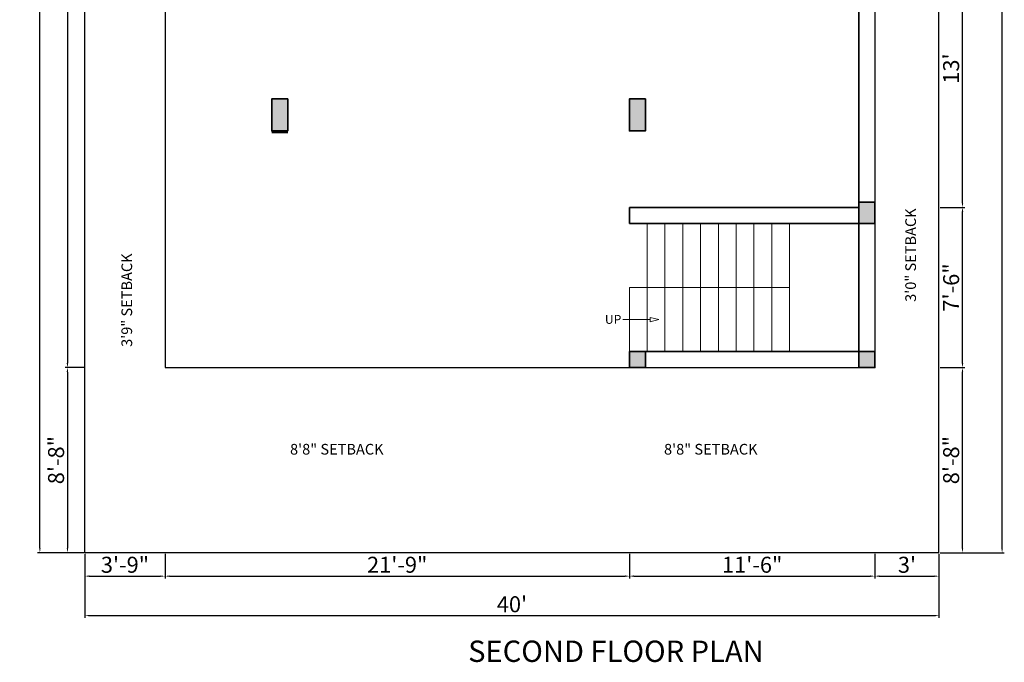
# Model space of a CAD drawing. Units: inches. Extents: x 3321 to 5237, y 11 to 1752.
# Tile 25 of 43: x 4649 to 5203, y 926 to 1287. Entities that reach past the tile are written whole.
import ezdxf

# ---------------------------------------------------------------- set-up
doc = ezdxf.new("R2010")
doc.units = ezdxf.units.IN
for name, color, linetype, lineweight in [('A-ANNO-DIMS', 2, 'Continuous', 18), ('A-ANNO-SYMB', 7, 'Continuous', 18), ('A-ANNO-TEXT', 7, 'Continuous', 18), ('A-ANNO-TITL', 7, 'Continuous', 25), ('A-COLS', 1, 'Continuous', 35), ('A-FLOR-EDGE', 7, 'Continuous', 25), ('A-FLOR-STRS', 7, 'Continuous', 18), ('A-WALL', 7, 'Continuous', 35), ('C-PROP', 7, 'Continuous', 30)]:
    doc.layers.add(name, color=color, linetype=linetype, lineweight=lineweight)
doc.styles.get("Standard").update_dxf_attribs({"font": 'arial.ttf'})
doc.dimstyles.new('ISO-25', dxfattribs={"dimtxt": 9, "dimasz": 2.5, "dimexe": 1.25, "dimexo": 0.625, "dimtad": 1, "dimdec": 1, "dimlunit": 3, "dimtxsty": 'Standard', "dimcen": 2.5, "dimclrd": 4, "dimclre": 4, "dimclrt": 256, "dimadec": 0, "dimazin": 0, "dimtfac": 1, "dimtdec": 1, "dimtmove": 0, "dimatfit": 3, "dimfxl": 1, "dimarcsym": 0})

# ---------------------------------------------------------------- blocks, each defined once
blk = doc.blocks.new('*D17')
at = {"layer": 'A-ANNO-DIMS', "color": 0, "lineweight": -2, "transparency": 16777216}
for p, q in [((4685.46, 1687.34), (4674.99, 1687.34)), ((4676.24, 1684.84), (4676.24, 1093.84)), ((4685.46, 1091.34), (4674.99, 1091.34))]:
    blk.add_line(p, q, dxfattribs=at)
at = {"layer": 'A-ANNO-DIMS', "color": 0, "transparency": 16777216}
for points in [[(4675.82, 1684.84), (4676.66, 1684.84), (4676.24, 1687.34)], [(4675.82, 1093.84), (4676.66, 1093.84), (4676.24, 1091.34)]]:
    blk.add_solid(points, dxfattribs=at)
at = {"layer": 'Defpoints', "color": 0, "transparency": 16777216}
for p in [(4686.08, 1687.34), (4676.24, 1091.34), (4686.08, 1091.34)]:
    blk.add_point(p, dxfattribs=at)
at = {"layer": 'A-ANNO-DIMS', "color": 0, "transparency": 16777216, "insert": (4671.02, 1389.34), "char_height": 9, "attachment_point": 5, "rotation": 90}
blk.add_mtext('49\'-8"', dxfattribs=at)
blk = doc.blocks.new('*D18')
at = {"layer": 'A-ANNO-DIMS', "color": 0, "lineweight": -2, "transparency": 16777216}
for p, q in [((4685.46, 1091.34), (4674.99, 1091.34)), ((4676.24, 1088.84), (4676.24, 989.84)), ((4685.46, 987.34), (4674.99, 987.34))]:
    blk.add_line(p, q, dxfattribs=at)
at = {"layer": 'A-ANNO-DIMS', "color": 0, "transparency": 16777216}
for points in [[(4675.82, 1088.84), (4676.66, 1088.84), (4676.24, 1091.34)], [(4675.82, 989.84), (4676.66, 989.84), (4676.24, 987.34)]]:
    blk.add_solid(points, dxfattribs=at)
at = {"layer": 'Defpoints', "color": 0, "transparency": 16777216}
for p in [(4686.08, 1091.34), (4676.24, 987.34), (4686.08, 987.34)]:
    blk.add_point(p, dxfattribs=at)
at = {"layer": 'A-ANNO-DIMS', "color": 0, "transparency": 16777216, "insert": (4671.02, 1039.34), "char_height": 9, "attachment_point": 5, "rotation": 90}
blk.add_mtext('8\'-8"', dxfattribs=at)
blk = doc.blocks.new('*D19')
at = {"layer": 'A-ANNO-DIMS', "color": 0, "lineweight": -2, "transparency": 16777216}
for p, q in [((5166.71, 1091.34), (5180.54, 1091.34)), ((5179.29, 989.84), (5179.29, 1088.84)), ((5166.71, 987.34), (5180.54, 987.34))]:
    blk.add_line(p, q, dxfattribs=at)
at = {"layer": 'A-ANNO-DIMS', "color": 0, "transparency": 16777216}
for points in [[(5178.88, 1088.84), (5179.71, 1088.84), (5179.29, 1091.34)], [(5178.88, 989.84), (5179.71, 989.84), (5179.29, 987.34)]]:
    blk.add_solid(points, dxfattribs=at)
at = {"layer": 'Defpoints', "color": 0, "transparency": 16777216}
for p in [(5166.08, 1091.34), (5179.29, 1091.34), (5166.08, 987.34)]:
    blk.add_point(p, dxfattribs=at)
at = {"layer": 'A-ANNO-DIMS', "color": 0, "transparency": 16777216, "insert": (5174.07, 1039.34), "char_height": 9, "attachment_point": 5, "rotation": 90}
blk.add_mtext('8\'-8"', dxfattribs=at)
blk = doc.blocks.new('*D20')
at = {"layer": 'A-ANNO-DIMS', "color": 0, "lineweight": -2, "transparency": 16777216}
for p, q in [((5166.71, 1181.34), (5180.54, 1181.34)), ((5179.29, 1093.84), (5179.29, 1178.84)), ((5166.71, 1091.34), (5180.54, 1091.34))]:
    blk.add_line(p, q, dxfattribs=at)
at = {"layer": 'A-ANNO-DIMS', "color": 0, "transparency": 16777216}
for points in [[(5178.88, 1178.84), (5179.71, 1178.84), (5179.29, 1181.34)], [(5178.88, 1093.84), (5179.71, 1093.84), (5179.29, 1091.34)]]:
    blk.add_solid(points, dxfattribs=at)
at = {"layer": 'Defpoints', "color": 0, "transparency": 16777216}
for p in [(5166.08, 1181.34), (5179.29, 1181.34), (5166.08, 1091.34)]:
    blk.add_point(p, dxfattribs=at)
at = {"layer": 'A-ANNO-DIMS', "color": 0, "transparency": 16777216, "insert": (5174.07, 1136.34), "char_height": 9, "attachment_point": 5, "rotation": 90}
blk.add_mtext('7\'-6"', dxfattribs=at)
blk = doc.blocks.new('*D21')
at = {"layer": 'A-ANNO-DIMS', "color": 0, "lineweight": -2, "transparency": 16777216}
for p, q in [((5166.71, 1337.34), (5180.54, 1337.34)), ((5179.29, 1183.84), (5179.29, 1334.84)), ((5166.71, 1181.34), (5180.54, 1181.34))]:
    blk.add_line(p, q, dxfattribs=at)
at = {"layer": 'A-ANNO-DIMS', "color": 0, "transparency": 16777216}
for points in [[(5178.88, 1334.84), (5179.71, 1334.84), (5179.29, 1337.34)], [(5178.88, 1183.84), (5179.71, 1183.84), (5179.29, 1181.34)]]:
    blk.add_solid(points, dxfattribs=at)
at = {"layer": 'Defpoints', "color": 0, "transparency": 16777216}
for p in [(5166.08, 1337.34), (5179.29, 1337.34), (5166.08, 1181.34)]:
    blk.add_point(p, dxfattribs=at)
at = {"layer": 'A-ANNO-DIMS', "color": 0, "transparency": 16777216, "insert": (5174.07, 1259.34), "char_height": 9, "attachment_point": 5, "rotation": 90}
blk.add_mtext("13'", dxfattribs=at)
blk = doc.blocks.new('*D24')
at = {"layer": 'A-ANNO-DIMS', "color": 0, "lineweight": -2, "transparency": 16777216}
for p, q in [((4686.08, 986.71), (4686.08, 972.9)), ((4731.08, 986.71), (4731.08, 972.9)), ((4688.58, 974.15), (4728.58, 974.15))]:
    blk.add_line(p, q, dxfattribs=at)
at = {"layer": 'A-ANNO-DIMS', "color": 0, "transparency": 16777216}
for points in [[(4688.58, 974.57), (4688.58, 973.74), (4686.08, 974.15)], [(4728.58, 974.57), (4728.58, 973.74), (4731.08, 974.15)]]:
    blk.add_solid(points, dxfattribs=at)
at = {"layer": 'Defpoints', "color": 0, "transparency": 16777216}
for p in [(4686.08, 987.34), (4731.08, 987.34), (4731.08, 974.15)]:
    blk.add_point(p, dxfattribs=at)
at = {"layer": 'A-ANNO-DIMS', "color": 0, "transparency": 16777216, "insert": (4708.58, 979.38), "char_height": 9, "attachment_point": 5}
blk.add_mtext('3\'-9"', dxfattribs=at)
blk = doc.blocks.new('*D25')
at = {"layer": 'A-ANNO-DIMS', "color": 0, "lineweight": -2, "transparency": 16777216}
for p, q in [((4731.08, 986.71), (4731.08, 972.9)), ((4992.08, 986.71), (4992.08, 972.9)), ((4733.58, 974.15), (4989.58, 974.15))]:
    blk.add_line(p, q, dxfattribs=at)
at = {"layer": 'A-ANNO-DIMS', "color": 0, "transparency": 16777216}
for points in [[(4733.58, 974.57), (4733.58, 973.74), (4731.08, 974.15)], [(4989.58, 974.57), (4989.58, 973.74), (4992.08, 974.15)]]:
    blk.add_solid(points, dxfattribs=at)
at = {"layer": 'Defpoints', "color": 0, "transparency": 16777216}
for p in [(4731.08, 987.34), (4992.08, 987.34), (4992.08, 974.15)]:
    blk.add_point(p, dxfattribs=at)
at = {"layer": 'A-ANNO-DIMS', "color": 0, "transparency": 16777216, "insert": (4861.58, 979.38), "char_height": 9, "attachment_point": 5}
blk.add_mtext('21\'-9"', dxfattribs=at)
blk = doc.blocks.new('*D26')
at = {"layer": 'A-ANNO-DIMS', "color": 0, "lineweight": -2, "transparency": 16777216}
for p, q in [((4992.08, 986.71), (4992.08, 972.9)), ((5130.08, 986.71), (5130.08, 972.9)), ((4994.58, 974.15), (5127.58, 974.15))]:
    blk.add_line(p, q, dxfattribs=at)
at = {"layer": 'A-ANNO-DIMS', "color": 0, "transparency": 16777216}
for points in [[(4994.58, 974.57), (4994.58, 973.74), (4992.08, 974.15)], [(5127.58, 974.57), (5127.58, 973.74), (5130.08, 974.15)]]:
    blk.add_solid(points, dxfattribs=at)
at = {"layer": 'Defpoints', "color": 0, "transparency": 16777216}
for p in [(4992.08, 987.34), (5130.08, 987.34), (5130.08, 974.15)]:
    blk.add_point(p, dxfattribs=at)
at = {"layer": 'A-ANNO-DIMS', "color": 0, "transparency": 16777216, "insert": (5061.08, 979.38), "char_height": 9, "attachment_point": 5}
blk.add_mtext('11\'-6"', dxfattribs=at)
blk = doc.blocks.new('*D27')
at = {"layer": 'A-ANNO-DIMS', "color": 0, "lineweight": -2, "transparency": 16777216}
for p, q in [((5130.08, 986.71), (5130.08, 972.9)), ((5166.08, 986.71), (5166.08, 972.9)), ((5132.58, 974.15), (5163.58, 974.15))]:
    blk.add_line(p, q, dxfattribs=at)
at = {"layer": 'A-ANNO-DIMS', "color": 0, "transparency": 16777216}
for points in [[(5132.58, 974.57), (5132.58, 973.74), (5130.08, 974.15)], [(5163.58, 974.57), (5163.58, 973.74), (5166.08, 974.15)]]:
    blk.add_solid(points, dxfattribs=at)
at = {"layer": 'Defpoints', "color": 0, "transparency": 16777216}
for p in [(5130.08, 987.34), (5166.08, 987.34), (5166.08, 974.15)]:
    blk.add_point(p, dxfattribs=at)
at = {"layer": 'A-ANNO-DIMS', "color": 0, "transparency": 16777216, "insert": (5148.08, 979.38), "char_height": 9, "attachment_point": 5}
blk.add_mtext("3'", dxfattribs=at)
blk = doc.blocks.new('*D28')
at = {"layer": 'A-ANNO-DIMS', "color": 0, "lineweight": -2, "transparency": 16777216}
for p, q in [((4686.08, 986.71), (4686.08, 950.73)), ((5166.08, 986.71), (5166.08, 950.73)), ((4688.58, 951.98), (5163.58, 951.98))]:
    blk.add_line(p, q, dxfattribs=at)
at = {"layer": 'A-ANNO-DIMS', "color": 0, "transparency": 16777216}
for points in [[(4688.58, 952.4), (4688.58, 951.56), (4686.08, 951.98)], [(5163.58, 952.4), (5163.58, 951.56), (5166.08, 951.98)]]:
    blk.add_solid(points, dxfattribs=at)
at = {"layer": 'Defpoints', "color": 0, "transparency": 16777216}
for p in [(4686.08, 987.34), (5166.08, 987.34), (5166.08, 951.98)]:
    blk.add_point(p, dxfattribs=at)
at = {"layer": 'A-ANNO-DIMS', "color": 0, "transparency": 16777216, "insert": (4926.08, 957.2), "char_height": 9, "attachment_point": 5}
blk.add_mtext("40'", dxfattribs=at)
blk = doc.blocks.new('*D29')
at = {"layer": 'A-ANNO-DIMS', "color": 0, "lineweight": -2, "transparency": 16777216}
for p, q in [((4685.46, 1707.34), (4659.51, 1707.34)), ((4660.76, 989.84), (4660.76, 1704.84)), ((4685.46, 987.34), (4659.51, 987.34))]:
    blk.add_line(p, q, dxfattribs=at)
at = {"layer": 'A-ANNO-DIMS', "color": 0, "transparency": 16777216}
for points in [[(4660.35, 1704.84), (4661.18, 1704.84), (4660.76, 1707.34)], [(4660.35, 989.84), (4661.18, 989.84), (4660.76, 987.34)]]:
    blk.add_solid(points, dxfattribs=at)
at = {"layer": 'Defpoints', "color": 0, "transparency": 16777216}
for p in [(4660.76, 1707.34), (4686.08, 1707.34), (4686.08, 987.34)]:
    blk.add_point(p, dxfattribs=at)
at = {"layer": 'A-ANNO-DIMS', "color": 0, "transparency": 16777216, "insert": (4655.54, 1347.34), "char_height": 9, "attachment_point": 5, "rotation": 90}
blk.add_mtext("60'", dxfattribs=at)
blk = doc.blocks.new('*D148')
at = {"layer": 'A-ANNO-DIMS', "color": 0, "lineweight": -2, "transparency": 16777216}
for p, q in [((5166.71, 1707.34), (5202.79, 1707.34)), ((5201.54, 989.84), (5201.54, 1704.84)), ((5166.71, 987.34), (5202.79, 987.34))]:
    blk.add_line(p, q, dxfattribs=at)
at = {"layer": 'A-ANNO-DIMS', "color": 0, "transparency": 16777216}
for points in [[(5201.12, 1704.84), (5201.96, 1704.84), (5201.54, 1707.34)], [(5201.12, 989.84), (5201.96, 989.84), (5201.54, 987.34)]]:
    blk.add_solid(points, dxfattribs=at)
at = {"layer": 'Defpoints', "color": 0, "transparency": 16777216}
for p in [(5166.08, 1707.34), (5201.54, 1707.34), (5166.08, 987.34)]:
    blk.add_point(p, dxfattribs=at)
at = {"layer": 'A-ANNO-DIMS', "color": 0, "transparency": 16777216, "insert": (5196.32, 1347.34), "char_height": 9, "attachment_point": 5, "rotation": 90}
blk.add_mtext("60'", dxfattribs=at)
blk = doc.blocks.new('COL-9X18-IN')
h = blk.add_hatch(color=256)
h.dxf.hatch_style = 1
h.paths.add_polyline_path([(9, 18), (0, 18), (0, 0), (9, 0)])
blk.add_lwpolyline([(0, 0), (9, 0), (9, 18), (0, 18)], close=True)
blk = doc.blocks.new('COL-9X12-FURN-PLAN')
h = blk.add_hatch(color=256)
h.dxf.hatch_style = 1
h.paths.add_polyline_path([(0, 12), (0, 0), (9, 0), (9, 12)])
blk.add_lwpolyline([(0, 0), (9, 0), (9, 12), (0, 12)], close=True)
blk = doc.blocks.new('COL-9X9-FURN-PLAN')
h = blk.add_hatch(color=256)
h.dxf.hatch_style = 1
h.paths.add_polyline_path([(9, 9), (0, 9), (0, 0), (9, 0)])
blk.add_lwpolyline([(0, 0), (9, 0), (9, 9), (0, 9)], close=True)
blk = doc.blocks.new('STAIR-RETURN-72IN')
for p, q in [((10, 72), (10, 0)), ((20, 72), (20, 0)), ((30, 72), (30, 0)), ((40, 72), (40, 0)), ((50, 72), (50, 0)), ((60, 72), (60, 0)), ((70, 72), (70, 0)), ((80, 72), (80, 0)), ((90, 72), (90, 0)), ((90, 36), (0, 36)), ((0, 36), (0, 0))]:
    blk.add_line(p, q)
blk = doc.blocks.new('STAIR-DIRECTION-ARROW')
blk.add_line((0, 1.22), (15.43, 1.22))
blk.add_lwpolyline([(20.27, 1.22), (15.43, 2.43), (15.43, 0)], close=True)
blk = doc.blocks.new('PROPERTY-40X60FT')
for p, q in [((0, 720), (480, 720)), ((0, 720), (0, 0)), ((480, 720), (480, 0)), ((0, 0), (480, 0))]:
    blk.add_line(p, q)

msp = doc.modelspace()

# ---------------------------------------------------------------- linework, layer by layer
at = {"layer": 'A-COLS'}
msp.add_line((4791.08, 1223.34), (4800.08, 1223.34), dxfattribs=at)
at = {"layer": 'A-FLOR-EDGE'}
for p, q in [((4731.08, 1687.34), (4731.08, 1091.34)), ((5130.08, 1687.34), (5130.08, 1091.34)), ((4731.08, 1091.34), (5130.08, 1091.34))]:
    msp.add_line(p, q, dxfattribs=at)
at = {"layer": 'A-WALL'}
for p, q in [((5121.08, 1337.34), (5121.08, 1181.34)), ((4992.08, 1181.34), (5121.08, 1181.34)), ((4992.08, 1181.34), (4992.08, 1172.34)), ((4992.08, 1172.34), (5121.08, 1172.34)), ((5121.08, 1172.34), (5121.08, 1100.34)), ((4992.08, 1100.34), (4992.08, 1091.34)), ((4992.08, 1100.34), (5121.08, 1100.34))]:
    msp.add_line(p, q, dxfattribs=at)

# ---------------------------------------------------------------- block references
at = {"layer": 'A-ANNO-SYMB'}
msp.add_blockref('STAIR-DIRECTION-ARROW', (4988.36, 1117.12), dxfattribs=at)
at = {"layer": 'A-COLS', "rotation": 180}
for p in [(4800.08, 1242.34), (5001.08, 1242.34)]:
    msp.add_blockref('COL-9X18-IN', p, dxfattribs=at)
at = {"layer": 'A-COLS'}
for name, p in [('COL-9X12-FURN-PLAN', (5121.08, 1172.34)), ('COL-9X9-FURN-PLAN', (4992.08, 1091.34)), ('COL-9X9-FURN-PLAN', (5121.08, 1091.34))]:
    msp.add_blockref(name, p, dxfattribs=at)
at = {"layer": 'A-FLOR-STRS'}
msp.add_blockref('STAIR-RETURN-72IN', (4992.08, 1100.34), dxfattribs=at)
at = {"layer": 'C-PROP', "rotation": 180}
msp.add_blockref('PROPERTY-40X60FT', (5166.08, 1707.34), dxfattribs=at)

# ---------------------------------------------------------------- texts
at = {"layer": 'A-ANNO-TEXT'}
msp.add_text('UP', height=5, dxfattribs=at).set_placement((4978.3, 1115.94))
at = {"layer": 'A-ANNO-TEXT', "char_height": 6, "attachment_point": 1, "rotation": 90}
for s, insert in [('3\'0" SETBACK', (5147.15, 1128.26)), ('3\'9" SETBACK', (4706.6, 1102.96))]:
    msp.add_mtext_dynamic_manual_height_columns(s, width=97.3114, gutter_width=25, heights=[0], dxfattribs=dict(at, insert=insert))
at = {"layer": 'A-ANNO-TEXT', "char_height": 6, "attachment_point": 1}
for insert in [(4801.35, 1048.46), (5011.54, 1048.46)]:
    msp.add_mtext_dynamic_manual_height_columns('8\'8" SETBACK', width=97.3114, gutter_width=25, heights=[0], dxfattribs=dict(at, insert=insert))
at = {"layer": 'A-ANNO-TITL', "insert": (4901.47, 937.95), "char_height": 12, "attachment_point": 1}
msp.add_mtext_dynamic_manual_height_columns('SECOND FLOOR PLAN', width=241.3793, gutter_width=25, heights=[0], dxfattribs=at)

# ---------------------------------------------------------------- dimensions: what is measured, and where the dimension line sits
at = {"layer": 'A-ANNO-DIMS'}
for base, p1, p2, angle, override, picture, middle in [((4660.76, 1707.34), (4686.08, 987.34), (4686.08, 1707.34), 90, {"dimclrd": 0, "dimclre": 0, "dimclrt": 0}, '*D29', (4655.54, 1347.34)), ((5201.54, 1707.34), (5166.08, 987.34), (5166.08, 1707.34), 270, {"dimclrd": 0, "dimclre": 0, "dimclrt": 0}, '*D148', (5196.32, 1347.34)), ((4676.24, 1091.34), (4686.08, 1687.34), (4686.08, 1091.34), 90, {"dimclrd": 0, "dimclre": 0, "dimclrt": 0}, '*D17', (4671.02, 1389.34)), ((5179.29, 1337.34), (5166.08, 1181.34), (5166.08, 1337.34), 90, {"dimclrd": 0, "dimclre": 0, "dimclrt": 0, "dimtmove": 1}, '*D21', (5174.07, 1259.34)), ((5179.29, 1181.34), (5166.08, 1091.34), (5166.08, 1181.34), 90, {"dimclrd": 0, "dimclre": 0, "dimclrt": 0, "dimtmove": 1}, '*D20', (5174.07, 1136.34)), ((4676.24, 987.34), (4686.08, 1091.34), (4686.08, 987.34), 90, {"dimclrd": 0, "dimclre": 0, "dimclrt": 0}, '*D18', (4671.02, 1039.34)), ((5179.29, 1091.34), (5166.08, 987.34), (5166.08, 1091.34), 90, {"dimclrd": 0, "dimclre": 0, "dimclrt": 0}, '*D19', (5174.07, 1039.34))]:
    dim = msp.add_linear_dim(base=base, p1=p1, p2=p2, angle=angle, dimstyle='ISO-25', override=override, dxfattribs=at)
    dim.commit()
    dim.dimension.update_dxf_attribs({"geometry": picture, "text_midpoint": middle})
for base, p1, p2, override, picture, middle in [((4731.08, 974.15), (4686.08, 987.34), (4731.08, 987.34), {"dimclrd": 0, "dimclre": 0, "dimclrt": 0}, '*D24', (4708.58, 979.38)), ((5166.08, 951.98), (4686.08, 987.34), (5166.08, 987.34), {"dimclrd": 0, "dimclre": 0, "dimclrt": 0}, '*D28', (4926.08, 957.2)), ((4992.08, 974.15), (4731.08, 987.34), (4992.08, 987.34), {"dimclrd": 0, "dimclre": 0, "dimclrt": 0, "dimtmove": 1}, '*D25', (4861.58, 979.38)), ((5130.08, 974.15), (4992.08, 987.34), (5130.08, 987.34), {"dimclrd": 0, "dimclre": 0, "dimclrt": 0, "dimtmove": 1}, '*D26', (5061.08, 979.38)), ((5166.08, 974.15), (5130.08, 987.34), (5166.08, 987.34), {"dimclrd": 0, "dimclre": 0, "dimclrt": 0, "dimtmove": 1}, '*D27', (5148.08, 979.38))]:
    dim = msp.add_linear_dim(base=base, p1=p1, p2=p2, dimstyle='ISO-25', override=override, dxfattribs=at)
    dim.commit()
    dim.dimension.update_dxf_attribs({"geometry": picture, "text_midpoint": middle})

doc.saveas('drawing.dxf')
